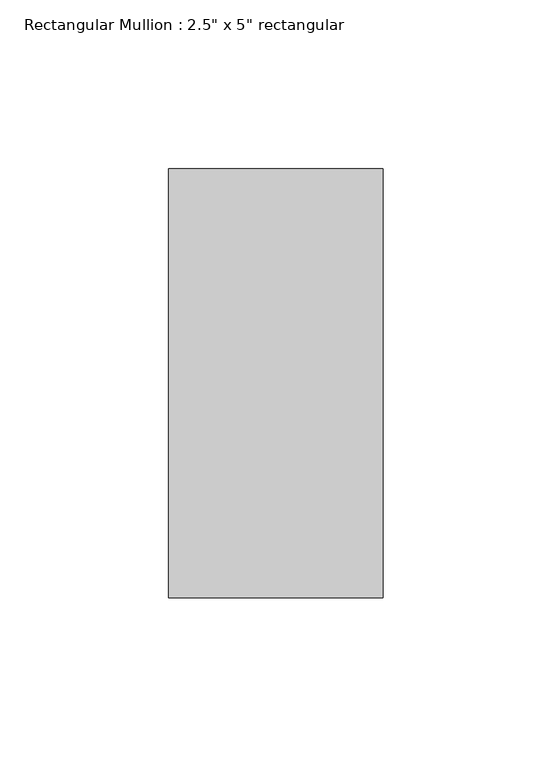
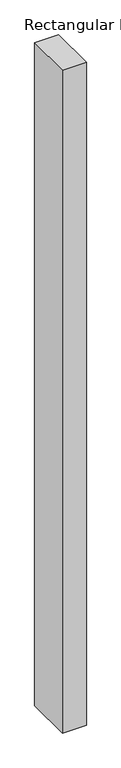
"""IFC4 building model written with IfcOpenShell, lengths in millimetres: member geometry."""

from ifc_helpers import new_model, si_unit, frame, origin, place, context, project, spatial, polyline, outline, extrude, source, transform, mapped, element, save


def member_18118615(model_context):
    return source(origin(), model_context, "Body", "SweptSolid", [
        extrude(outline(polyline([(31.75, 63.5), (31.75, -63.5), (-31.75, -63.5), (-31.75, 63.5), (31.75, 63.5)])), frame((0.0, 0.0, -1855.6083676), z_axis=(0.0, 0.0, 1.0), x_axis=(1.0, 0.0, 0.0)), (0.0, 0.0, 1.0), 1855.6083676),
    ])


if __name__ == "__main__":
    model = new_model("IFC4")
    model_context = context("Model", 3, world=origin())
    ifc_project = project(units=[si_unit("LENGTHUNIT", "METRE", prefix="MILLI")], contexts=[model_context])
    site = spatial("IfcSite", under=ifc_project)
    building = spatial("IfcBuilding", under=site)
    placement = place(None, origin())
    member_shape = member_18118615(model_context)
    element("IfcMember", 1, ObjectType="Rectangular Mullion : 2.5\" x 5\" rectangular", at=placement, inside=building, context=model_context, shape_type="MappedRepresentation", body=[
        mapped(member_shape, transform((0.0, 0.0, 0.0), x_axis=(1.0, 0.0, 0.0), y_axis=(0.0, 1.0, 0.0), z_axis=(0.0, 0.0, 1.0))),
    ])
    save(model, "model.ifc")

# Revit data of these elements
# Type "Rectangular Mullion : 2.5\" x 5\" rectangular"
#   built-in parameter 1007304 = 0.416667 (stored number, unit not read)
#   built-in parameter 1007301 = 0.104167 (stored number, unit not read)
#   built-in parameter 1007300 = 0.104167 (stored number, unit not read)
# Element 1 (IfcMember, "Rectangular Mullion : 2.5\" x 5\" rectangular")
#   Materials on its faces: "Aluminum"
# Materials
#   "Aluminum": class "Metal", colour RGB 247 247 247, transparency 0, Description = "Aluminum 6061", Cost = 0
